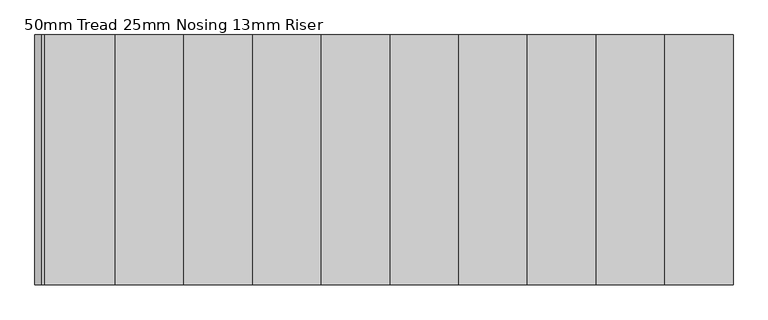
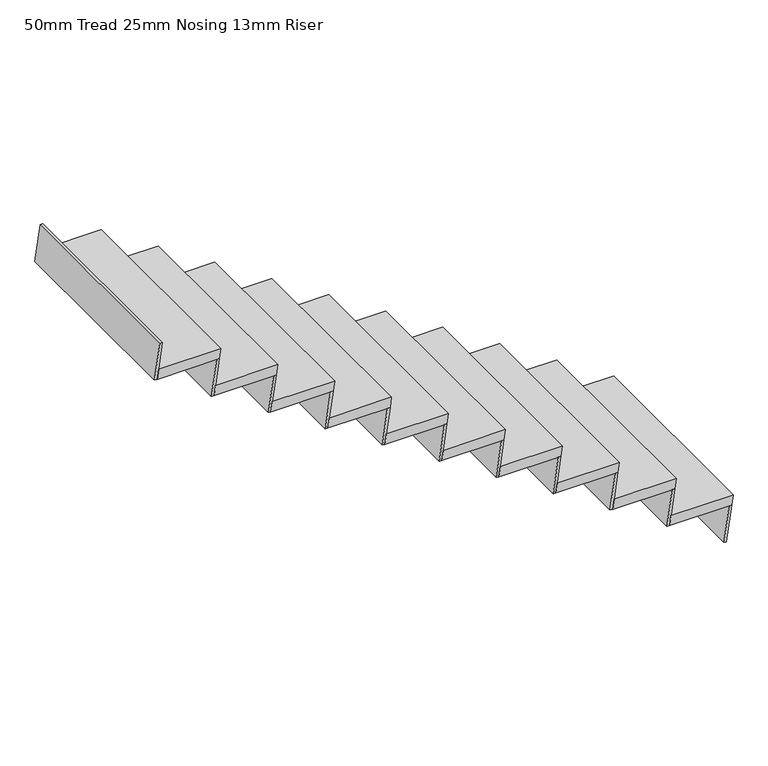
"""IFC4 building model written with IfcOpenShell, lengths in millimetres: stair flight geometry, 50mm Tread 25mm Nosing 13mm Riser."""

from ifc_helpers import new_model, si_unit, frame, origin, place, context, project, spatial, polyline, outline, extrude, source, transform, mapped, element, save


def stair_flight_50mm_tread_25mm_nosing_13mm_riser_9fd7d1ab(model_context):
    return source(origin(), model_context, "Body", "SweptSolid", [
        extrude(outline(polyline([(1255.0588235, 12375.7864069), (1255.0588235, 12075.7864069), (1205.0588235, 12068.8146221), (1205.0588235, 12368.8146221), (1255.0588235, 12375.7864069)])), frame((0.0, -1011.9101069, 0.0), z_axis=(0.0, 1.0, 0.0), x_axis=(0.0, 0.0, 1.0)), (0.0, 0.0, 1.0), 1000.0257812),
        extrude(outline(polyline([(1205.0588235, 12368.8146221), (1205.0588235, 12356.1936926), (1025.7647059, 12331.1936926), (1025.7647059, 12343.8146221), (1205.0588235, 12368.8146221)])), frame((0.0, -1011.9101069, 0.0), z_axis=(0.0, 1.0, 0.0), x_axis=(0.0, 0.0, 1.0)), (0.0, 0.0, 1.0), 1000.0257812),
        extrude(outline(polyline([(1384.3529412, 12093.8146221), (1384.3529412, 12081.1936926), (1205.0588235, 12056.1936926), (1205.0588235, 12068.8146221), (1384.3529412, 12093.8146221)])), frame((0.0, -1011.9101069, 0.0), z_axis=(0.0, 1.0, 0.0), x_axis=(0.0, 0.0, 1.0)), (0.0, 0.0, 1.0), 1000.0257813),
        extrude(outline(polyline([(1434.3529412, 12100.7864069), (1434.3529412, 11800.7864069), (1384.3529412, 11793.8146221), (1384.3529412, 12093.8146221), (1434.3529412, 12100.7864069)])), frame((0.0, -1011.9101069, 0.0), z_axis=(0.0, 1.0, 0.0), x_axis=(0.0, 0.0, 1.0)), (0.0, 0.0, 1.0), 1000.0257812),
        extrude(outline(polyline([(1563.6470588, 11818.8146221), (1563.6470588, 11806.1936926), (1384.3529412, 11781.1936926), (1384.3529412, 11793.8146221), (1563.6470588, 11818.8146221)])), frame((0.0, -1011.9101069, 0.0), z_axis=(0.0, 1.0, 0.0), x_axis=(0.0, 0.0, 1.0)), (0.0, 0.0, 1.0), 1000.0257812),
        extrude(outline(polyline([(1613.6470588, 11825.7864069), (1613.6470588, 11525.7864069), (1563.6470588, 11518.8146221), (1563.6470588, 11818.8146221), (1613.6470588, 11825.7864069)])), frame((0.0, -1011.9101069, 0.0), z_axis=(0.0, 1.0, 0.0), x_axis=(0.0, 0.0, 1.0)), (0.0, 0.0, 1.0), 1000.0257812),
        extrude(outline(polyline([(1742.9411765, 11543.8146221), (1742.9411765, 11531.1936926), (1563.6470588, 11506.1936926), (1563.6470588, 11518.8146221), (1742.9411765, 11543.8146221)])), frame((0.0, -1011.9101069, 0.0), z_axis=(0.0, 1.0, 0.0), x_axis=(0.0, 0.0, 1.0)), (0.0, 0.0, 1.0), 1000.0257812),
        extrude(outline(polyline([(1792.9411765, 11550.7864069), (1792.9411765, 11250.7864069), (1742.9411765, 11243.8146221), (1742.9411765, 11543.8146221), (1792.9411765, 11550.7864069)])), frame((0.0, -1011.9101069, 0.0), z_axis=(0.0, 1.0, 0.0), x_axis=(0.0, 0.0, 1.0)), (0.0, 0.0, 1.0), 1000.0257812),
        extrude(outline(polyline([(1922.2352941, 11268.8146221), (1922.2352941, 11256.1936926), (1742.9411765, 11231.1936926), (1742.9411765, 11243.8146221), (1922.2352941, 11268.8146221)])), frame((0.0, -1011.9101069, 0.0), z_axis=(0.0, 1.0, 0.0), x_axis=(0.0, 0.0, 1.0)), (0.0, 0.0, 1.0), 1000.0257813),
        extrude(outline(polyline([(1972.2352941, 11275.7864069), (1972.2352941, 10975.7864069), (1922.2352941, 10968.8146221), (1922.2352941, 11268.8146221), (1972.2352941, 11275.7864069)])), frame((0.0, -1011.9101069, 0.0), z_axis=(0.0, 1.0, 0.0), x_axis=(0.0, 0.0, 1.0)), (0.0, 0.0, 1.0), 1000.0257812),
        extrude(outline(polyline([(2101.5294118, 10993.8146221), (2101.5294118, 10981.1936926), (1922.2352941, 10956.1936926), (1922.2352941, 10968.8146221), (2101.5294118, 10993.8146221)])), frame((0.0, -1011.9101069, 0.0), z_axis=(0.0, 1.0, 0.0), x_axis=(0.0, 0.0, 1.0)), (0.0, 0.0, 1.0), 1000.0257812),
        extrude(outline(polyline([(2151.5294118, 11000.7864069), (2151.5294118, 10700.7864069), (2101.5294118, 10693.8146221), (2101.5294118, 10993.8146221), (2151.5294118, 11000.7864069)])), frame((0.0, -1011.9101069, 0.0), z_axis=(0.0, 1.0, 0.0), x_axis=(0.0, 0.0, 1.0)), (0.0, 0.0, 1.0), 1000.0257812),
        extrude(outline(polyline([(2280.8235294, 10718.8146221), (2280.8235294, 10706.1936926), (2101.5294118, 10681.1936926), (2101.5294118, 10693.8146221), (2280.8235294, 10718.8146221)])), frame((0.0, -1011.9101069, 0.0), z_axis=(0.0, 1.0, 0.0), x_axis=(0.0, 0.0, 1.0)), (0.0, 0.0, 1.0), 1000.0257812),
        extrude(outline(polyline([(2330.8235294, 10725.7864069), (2330.8235294, 10425.7864069), (2280.8235294, 10418.8146221), (2280.8235294, 10718.8146221), (2330.8235294, 10725.7864069)])), frame((0.0, -1011.9101069, 0.0), z_axis=(0.0, 1.0, 0.0), x_axis=(0.0, 0.0, 1.0)), (0.0, 0.0, 1.0), 1000.0257812),
        extrude(outline(polyline([(2460.1176471, 10443.8146221), (2460.1176471, 10431.1936926), (2280.8235294, 10406.1936926), (2280.8235294, 10418.8146221), (2460.1176471, 10443.8146221)])), frame((0.0, -1011.9101069, 0.0), z_axis=(0.0, 1.0, 0.0), x_axis=(0.0, 0.0, 1.0)), (0.0, 0.0, 1.0), 1000.0257813),
        extrude(outline(polyline([(2510.1176471, 10450.7864069), (2510.1176471, 10150.7864069), (2460.1176471, 10143.8146221), (2460.1176471, 10443.8146221), (2510.1176471, 10450.7864069)])), frame((0.0, -1011.9101069, 0.0), z_axis=(0.0, 1.0, 0.0), x_axis=(0.0, 0.0, 1.0)), (0.0, 0.0, 1.0), 1000.0257812),
        extrude(outline(polyline([(2639.4117647, 10168.8146221), (2639.4117647, 10156.1936926), (2460.1176471, 10131.1936926), (2460.1176471, 10143.8146221), (2639.4117647, 10168.8146221)])), frame((0.0, -1011.9101069, 0.0), z_axis=(0.0, 1.0, 0.0), x_axis=(0.0, 0.0, 1.0)), (0.0, 0.0, 1.0), 1000.0257812),
        extrude(outline(polyline([(2689.4117647, 10175.7864069), (2689.4117647, 9875.7864069), (2639.4117647, 9868.8146221), (2639.4117647, 10168.8146221), (2689.4117647, 10175.7864069)])), frame((0.0, -1011.9101069, 0.0), z_axis=(0.0, 1.0, 0.0), x_axis=(0.0, 0.0, 1.0)), (0.0, 0.0, 1.0), 1000.0257812),
        extrude(outline(polyline([(2818.7058824, 9893.8146221), (2818.7058824, 9881.1936926), (2639.4117647, 9856.1936926), (2639.4117647, 9868.8146221), (2818.7058824, 9893.8146221)])), frame((0.0, -1011.9101069, 0.0), z_axis=(0.0, 1.0, 0.0), x_axis=(0.0, 0.0, 1.0)), (0.0, 0.0, 1.0), 1000.0257812),
        extrude(outline(polyline([(2868.7058824, 9900.7864069), (2868.7058824, 9600.7864069), (2818.7058824, 9593.8146221), (2818.7058824, 9893.8146221), (2868.7058824, 9900.7864069)])), frame((0.0, -1011.9101069, 0.0), z_axis=(0.0, 1.0, 0.0), x_axis=(0.0, 0.0, 1.0)), (0.0, 0.0, 1.0), 1000.0257812),
        extrude(outline(polyline([(2998.0, 9618.8146221), (2998.0, 9606.1936926), (2818.7058824, 9581.1936926), (2818.7058824, 9593.8146221), (2998.0, 9618.8146221)])), frame((0.0, -1011.9101069, 0.0), z_axis=(0.0, 1.0, 0.0), x_axis=(0.0, 0.0, 1.0)), (0.0, 0.0, 1.0), 1000.0257812),
    ])


if __name__ == "__main__":
    model = new_model("IFC4")
    model_context = context("Model", 3, world=origin())
    ifc_project = project(units=[si_unit("LENGTHUNIT", "METRE", prefix="MILLI")], contexts=[model_context])
    site = spatial("IfcSite", under=ifc_project)
    building = spatial("IfcBuilding", under=site)
    placement = place(None, origin())
    stair_flight_50mm_tread_25mm_nosing_13mm_riser_shape = stair_flight_50mm_tread_25mm_nosing_13mm_riser_9fd7d1ab(model_context)
    element("IfcStairFlight", 1, ObjectType="50mm Tread 25mm Nosing 13mm Riser", at=placement, inside=building, context=model_context, shape_type="MappedRepresentation", body=[
        mapped(stair_flight_50mm_tread_25mm_nosing_13mm_riser_shape, transform((0.0, 0.0, 0.0), x_axis=(1.0, 0.0, 0.0), y_axis=(0.0, 1.0, 0.0), z_axis=(0.0, 0.0, 1.0))),
    ])
    save(model, "model.ifc")
